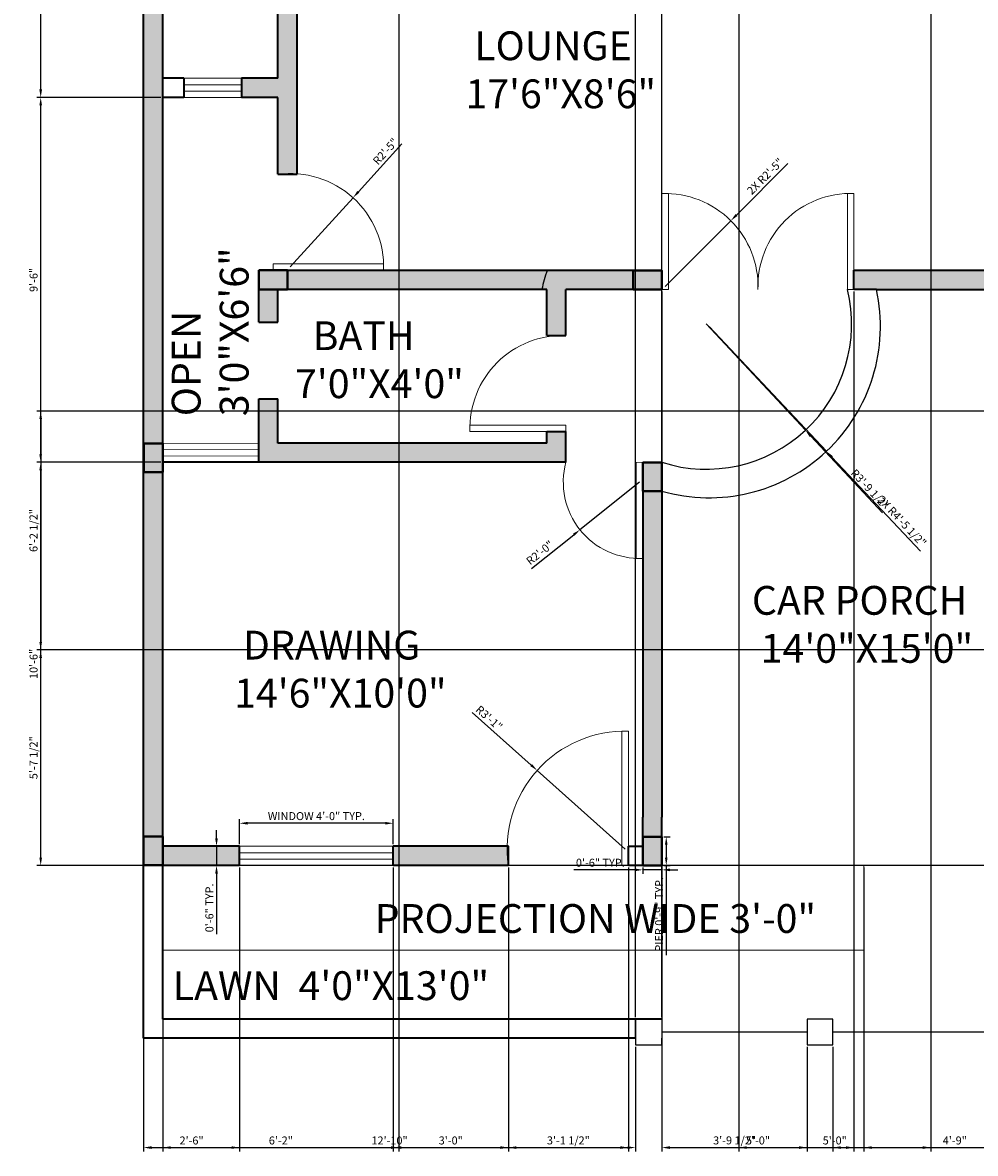
# Model space of a CAD drawing. Units: inches. Extents: x 5276 to 5736, y 3292 to 3966.
# Tile 1 of 3: x 5276 to 5574, y 3292 to 3646. Entities that reach past the tile are written whole.
import ezdxf

# ---------------------------------------------------------------- set-up
doc = ezdxf.new("R2010")
doc.units = ezdxf.units.IN
for name, color, linetype, lineweight in [('A-ANNO-DIMS', 2, 'Continuous', 18), ('A-ANNO-TEXT', 7, 'Continuous', 18), ('A-AREA-IDEN', 7, 'Continuous', 18), ('A-COLS', 7, 'Continuous', 40), ('A-DOOR', 3, 'Continuous', 18), ('A-FLOR', 7, 'Continuous', 25), ('A-GLAZ', 4, 'Continuous', 18), ('A-ROOF', 9, 'Continuous', 18), ('A-SITE-GATE', 7, 'Continuous', 25), ('A-WALL', 7, 'Continuous', 35)]:
    doc.layers.add(name, color=color, linetype=linetype, lineweight=lineweight)
doc.layers.add('A-COLS-PATT', color=244, linetype='Continuous', lineweight=13, true_color=0x991b1e)
doc.layers.add('A-WALL-PATT', color=141, linetype='Continuous', lineweight=13, true_color=0xadddf7)
doc.styles.get("Standard").update_dxf_attribs({"font": 'arial.ttf'})
doc.dimstyles.new('ISO-25', dxfattribs={"dimtxt": 2.5, "dimasz": 2.5, "dimexe": 1.25, "dimexo": 0.625, "dimtad": 1, "dimlunit": 3, "dimtxsty": 'Standard', "dimcen": 2.5, "dimadec": 0, "dimazin": 0, "dimtfac": 1, "dimtmove": 0, "dimatfit": 3, "dimfxl": 1, "dimarcsym": 0})

# ---------------------------------------------------------------- blocks, each defined once
blk = doc.blocks.new('PIER-6X9')
for p, q in [((0, 9), (6, 9)), ((0, 0), (0, 9)), ((6, 9), (6, 0)), ((6, 0), (0, 0))]:
    blk.add_line(p, q)
blk = doc.blocks.new('DOOR-SWING-30')
for p, q in [((0, 30), (-2, 30)), ((-2, 30), (-2, 0)), ((0, 0), (0, 30)), ((-2, 0), (0, 0))]:
    blk.add_line(p, q)
blk.add_arc((-1, 1), 29.02, 88.0251, 181.9749)
blk = doc.blocks.new('WINDOW-48X6')
for p, q in [((0, 6), (0, 0)), ((48, 6), (0, 6)), ((48, 4), (0, 4)), ((48, 0), (48, 6)), ((48, 2), (0, 2)), ((0, 0), (48, 0))]:
    blk.add_line(p, q)
blk = doc.blocks.new('*D22')
at = {"layer": 'A-ANNO-DIMS', "color": 0, "lineweight": -2, "transparency": 16777216}
for p, q in [((5476.74, 3391.24), (5478.72, 3391.24)), ((5477.47, 3388.74), (5477.47, 3384.74)), ((5476.74, 3382.24), (5478.72, 3382.24)), ((5477.47, 3382.24), (5477.47, 3354.25))]:
    blk.add_line(p, q, dxfattribs=at)
at = {"layer": 'A-ANNO-DIMS', "color": 0, "transparency": 16777216}
for points in [[(5477.05, 3388.74), (5477.88, 3388.74), (5477.47, 3391.24)], [(5477.05, 3384.74), (5477.88, 3384.74), (5477.47, 3382.24)]]:
    blk.add_solid(points, dxfattribs=at)
at = {"layer": 'Defpoints', "color": 0, "transparency": 16777216}
for p in [(5476.12, 3391.24), (5476.12, 3382.24), (5477.47, 3382.24)]:
    blk.add_point(p, dxfattribs=at)
at = {"layer": 'A-ANNO-DIMS', "color": 0, "transparency": 16777216, "insert": (5475.56, 3367), "char_height": 2.5, "attachment_point": 5, "rotation": 90}
blk.add_mtext('PIER 0\'-9" TYP.', dxfattribs=at)
blk = doc.blocks.new('*D23')
at = {"layer": 'A-ANNO-DIMS', "color": 0, "lineweight": -2, "transparency": 16777216}
for p, q in [((5467.62, 3380.89), (5448.63, 3380.89)), ((5470.12, 3381.61), (5470.12, 3379.64)), ((5476.12, 3380.89), (5470.12, 3380.89)), ((5476.12, 3381.61), (5476.12, 3379.64)), ((5478.62, 3380.89), (5481.12, 3380.89))]:
    blk.add_line(p, q, dxfattribs=at)
at = {"layer": 'A-ANNO-DIMS', "color": 0, "transparency": 16777216}
for points in [[(5467.62, 3381.31), (5467.62, 3380.47), (5470.12, 3380.89)], [(5478.62, 3381.31), (5478.62, 3380.47), (5476.12, 3380.89)]]:
    blk.add_solid(points, dxfattribs=at)
at = {"layer": 'Defpoints', "color": 0, "transparency": 16777216}
for p in [(5470.12, 3382.24), (5476.12, 3382.24), (5470.12, 3380.89)]:
    blk.add_point(p, dxfattribs=at)
at = {"layer": 'A-ANNO-DIMS', "color": 0, "transparency": 16777216, "insert": (5456.87, 3382.79), "char_height": 2.5, "attachment_point": 5}
blk.add_mtext('0\'-6" TYP.', dxfattribs=at)
blk = doc.blocks.new('*D28')
at = {"layer": 'A-ANNO-DIMS', "color": 0, "lineweight": -2, "transparency": 16777216}
for p, q in [((5344.13, 3388.87), (5344.13, 3396.7)), ((5392.13, 3388.87), (5392.13, 3396.7)), ((5389.63, 3395.45), (5346.63, 3395.45))]:
    blk.add_line(p, q, dxfattribs=at)
at = {"layer": 'A-ANNO-DIMS', "color": 0, "transparency": 16777216}
for points in [[(5346.63, 3395.87), (5346.63, 3395.03), (5344.13, 3395.45)], [(5389.63, 3395.87), (5389.63, 3395.03), (5392.13, 3395.45)]]:
    blk.add_solid(points, dxfattribs=at)
at = {"layer": 'Defpoints', "color": 0, "transparency": 16777216}
for p in [(5344.13, 3395.45), (5344.13, 3388.25), (5392.13, 3388.25)]:
    blk.add_point(p, dxfattribs=at)
at = {"layer": 'A-ANNO-DIMS', "color": 0, "transparency": 16777216, "insert": (5368.13, 3397.37), "char_height": 2.5, "attachment_point": 5}
blk.add_mtext('WINDOW 4\'-0" TYP.', dxfattribs=at)
blk = doc.blocks.new('*D29')
at = {"layer": 'A-ANNO-DIMS', "color": 0, "lineweight": -2, "transparency": 16777216}
for p, q in [((5336.93, 3390.75), (5336.93, 3393.25)), ((5343.5, 3388.25), (5335.68, 3388.25)), ((5336.93, 3388.25), (5336.93, 3382.25)), ((5343.5, 3382.25), (5335.68, 3382.25)), ((5336.93, 3379.75), (5336.93, 3360.76))]:
    blk.add_line(p, q, dxfattribs=at)
at = {"layer": 'A-ANNO-DIMS', "color": 0, "transparency": 16777216}
for points in [[(5336.51, 3390.75), (5337.34, 3390.75), (5336.93, 3388.25)], [(5336.51, 3379.75), (5337.34, 3379.75), (5336.93, 3382.25)]]:
    blk.add_solid(points, dxfattribs=at)
at = {"layer": 'Defpoints', "color": 0, "transparency": 16777216}
for p in [(5344.13, 3388.25), (5336.93, 3382.25), (5344.13, 3382.25)]:
    blk.add_point(p, dxfattribs=at)
at = {"layer": 'A-ANNO-DIMS', "color": 0, "transparency": 16777216, "insert": (5335.03, 3369), "char_height": 2.5, "attachment_point": 5, "rotation": 90}
blk.add_mtext('0\'-6" TYP.', dxfattribs=at)
blk = doc.blocks.new('*D30')
at = {"layer": 'A-ANNO-DIMS', "color": 0, "lineweight": -2, "transparency": 16777216}
for p, q in [((5314.13, 3327.62), (5314.13, 3292.85)), ((5467.88, 3325.62), (5467.88, 3292.85)), ((5316.63, 3294.1), (5465.38, 3294.1))]:
    blk.add_line(p, q, dxfattribs=at)
at = {"layer": 'A-ANNO-DIMS', "color": 0, "transparency": 16777216}
for points in [[(5316.63, 3294.52), (5316.63, 3293.68), (5314.13, 3294.1)], [(5465.38, 3294.52), (5465.38, 3293.68), (5467.88, 3294.1)]]:
    blk.add_solid(points, dxfattribs=at)
at = {"layer": 'Defpoints', "color": 0, "transparency": 16777216}
for p in [(5314.13, 3328.25), (5467.88, 3326.25), (5467.88, 3294.1)]:
    blk.add_point(p, dxfattribs=at)
at = {"layer": 'A-ANNO-DIMS', "color": 0, "transparency": 16777216, "insert": (5391, 3296), "char_height": 2.5, "attachment_point": 5}
blk.add_mtext('12\'-10"', dxfattribs=at)
blk = doc.blocks.new('*D31')
at = {"layer": 'A-ANNO-DIMS', "color": 0, "lineweight": -2, "transparency": 16777216}
for p, q in [((5476.13, 3325.62), (5476.13, 3292.85)), ((5521.5, 3325.62), (5521.5, 3292.85)), ((5478.63, 3294.1), (5519, 3294.1))]:
    blk.add_line(p, q, dxfattribs=at)
at = {"layer": 'A-ANNO-DIMS', "color": 0, "transparency": 16777216}
for points in [[(5478.63, 3294.52), (5478.63, 3293.68), (5476.13, 3294.1)], [(5519, 3294.52), (5519, 3293.68), (5521.5, 3294.1)]]:
    blk.add_solid(points, dxfattribs=at)
at = {"layer": 'Defpoints', "color": 0, "transparency": 16777216}
for p in [(5476.13, 3326.25), (5521.5, 3326.25), (5521.5, 3294.1)]:
    blk.add_point(p, dxfattribs=at)
at = {"layer": 'A-ANNO-DIMS', "color": 0, "transparency": 16777216, "insert": (5498.82, 3296.02), "char_height": 2.5, "attachment_point": 5}
blk.add_mtext('3\'-9 1/2"', dxfattribs=at)
blk = doc.blocks.new('*D32')
at = {"layer": 'A-ANNO-DIMS', "color": 0, "lineweight": -2, "transparency": 16777216}
for p, q in [((5529.5, 3325.62), (5529.5, 3292.85)), ((5672.13, 3325.62), (5672.13, 3292.85)), ((5532, 3294.1), (5669.63, 3294.1))]:
    blk.add_line(p, q, dxfattribs=at)
at = {"layer": 'A-ANNO-DIMS', "color": 0, "transparency": 16777216}
for points in [[(5532, 3294.52), (5532, 3293.68), (5529.5, 3294.1)], [(5669.63, 3294.52), (5669.63, 3293.68), (5672.13, 3294.1)]]:
    blk.add_solid(points, dxfattribs=at)
at = {"layer": 'Defpoints', "color": 0, "transparency": 16777216}
for p in [(5529.5, 3326.25), (5672.13, 3326.25), (5672.13, 3294.1)]:
    blk.add_point(p, dxfattribs=at)
at = {"layer": 'A-ANNO-DIMS', "color": 0, "transparency": 16777216, "insert": (5600.82, 3296.02), "char_height": 2.5, "attachment_point": 5}
blk.add_mtext('11\'-10 1/2"', dxfattribs=at)
blk = doc.blocks.new('*D33')
at = {"layer": 'A-ANNO-DIMS', "color": 0, "lineweight": -2, "transparency": 16777216}
for p, q in [((5467.88, 3334.87), (5467.88, 3961.65)), ((5476.13, 3334.87), (5476.13, 3961.65)), ((5470.38, 3960.4), (5473.63, 3960.4)), ((5476.13, 3960.4), (5492.35, 3960.4))]:
    blk.add_line(p, q, dxfattribs=at)
at = {"layer": 'A-ANNO-DIMS', "color": 0, "transparency": 16777216}
for points in [[(5470.38, 3960.82), (5470.38, 3959.98), (5467.88, 3960.4)], [(5473.63, 3960.82), (5473.63, 3959.98), (5476.13, 3960.4)]]:
    blk.add_solid(points, dxfattribs=at)
at = {"layer": 'Defpoints', "color": 0, "transparency": 16777216}
for p in [(5476.13, 3960.4), (5467.88, 3334.25), (5476.13, 3334.25)]:
    blk.add_point(p, dxfattribs=at)
at = {"layer": 'A-ANNO-DIMS', "color": 0, "transparency": 16777216, "insert": (5485.49, 3962.32), "char_height": 2.5, "attachment_point": 5}
blk.add_mtext('0\'-8 1/2"', dxfattribs=at)
blk = doc.blocks.new('*D36')
at = {"layer": 'A-ANNO-DIMS', "color": 0, "lineweight": -2, "transparency": 16777216}
for p, q in [((5319.5, 3508.25), (5280.73, 3508.25)), ((5281.98, 3384.75), (5281.98, 3505.75)), ((5319.5, 3382.25), (5280.73, 3382.25))]:
    blk.add_line(p, q, dxfattribs=at)
at = {"layer": 'A-ANNO-DIMS', "color": 0, "transparency": 16777216}
for points in [[(5281.56, 3505.75), (5282.39, 3505.75), (5281.98, 3508.25)], [(5281.56, 3384.75), (5282.39, 3384.75), (5281.98, 3382.25)]]:
    blk.add_solid(points, dxfattribs=at)
at = {"layer": 'Defpoints', "color": 0, "transparency": 16777216}
for p in [(5281.98, 3508.25), (5320.13, 3508.25), (5320.13, 3382.25)]:
    blk.add_point(p, dxfattribs=at)
at = {"layer": 'A-ANNO-DIMS', "color": 0, "transparency": 16777216, "insert": (5280.08, 3445.25), "char_height": 2.5, "attachment_point": 5, "rotation": 90}
blk.add_mtext('10\'-6"', dxfattribs=at)
blk = doc.blocks.new('*D37')
at = {"layer": 'A-ANNO-DIMS', "color": 0, "lineweight": -2, "transparency": 16777216}
for p, q in [((5319.5, 3622.25), (5280.73, 3622.25)), ((5281.98, 3510.75), (5281.98, 3619.75)), ((5319.5, 3508.25), (5280.73, 3508.25))]:
    blk.add_line(p, q, dxfattribs=at)
at = {"layer": 'A-ANNO-DIMS', "color": 0, "transparency": 16777216}
for points in [[(5281.56, 3619.75), (5282.39, 3619.75), (5281.98, 3622.25)], [(5281.56, 3510.75), (5282.39, 3510.75), (5281.98, 3508.25)]]:
    blk.add_solid(points, dxfattribs=at)
at = {"layer": 'Defpoints', "color": 0, "transparency": 16777216}
for p in [(5281.98, 3622.25), (5320.13, 3622.25), (5320.13, 3508.25)]:
    blk.add_point(p, dxfattribs=at)
at = {"layer": 'A-ANNO-DIMS', "color": 0, "transparency": 16777216, "insert": (5280.08, 3565.25), "char_height": 2.5, "attachment_point": 5, "rotation": 90}
blk.add_mtext('9\'-6"', dxfattribs=at)
blk = doc.blocks.new('*D38')
at = {"layer": 'A-ANNO-DIMS', "color": 0, "lineweight": -2, "transparency": 16777216}
for p, q in [((5319.5, 3730.25), (5280.73, 3730.25)), ((5281.98, 3624.75), (5281.98, 3727.75)), ((5319.5, 3622.25), (5280.73, 3622.25))]:
    blk.add_line(p, q, dxfattribs=at)
at = {"layer": 'A-ANNO-DIMS', "color": 0, "transparency": 16777216}
for points in [[(5281.56, 3727.75), (5282.39, 3727.75), (5281.98, 3730.25)], [(5281.56, 3624.75), (5282.39, 3624.75), (5281.98, 3622.25)]]:
    blk.add_solid(points, dxfattribs=at)
at = {"layer": 'Defpoints', "color": 0, "transparency": 16777216}
for p in [(5281.98, 3730.25), (5320.13, 3730.25), (5320.13, 3622.25)]:
    blk.add_point(p, dxfattribs=at)
at = {"layer": 'A-ANNO-DIMS', "color": 0, "transparency": 16777216, "insert": (5280.08, 3676.25), "char_height": 2.5, "attachment_point": 5, "rotation": 90}
blk.add_mtext('9\'-0"', dxfattribs=at)
blk = doc.blocks.new('*D41')
at = {"layer": 'A-ANNO-DIMS', "color": 0, "lineweight": -2, "transparency": 16777216}
for p, q in [((5476.13, 3382.87), (5476.13, 3961.65)), ((5596.12, 3382.87), (5596.12, 3961.65)), ((5478.63, 3960.4), (5593.62, 3960.4))]:
    blk.add_line(p, q, dxfattribs=at)
at = {"layer": 'A-ANNO-DIMS', "color": 0, "transparency": 16777216}
for points in [[(5478.63, 3960.82), (5478.63, 3959.98), (5476.13, 3960.4)], [(5593.62, 3960.82), (5593.62, 3959.98), (5596.12, 3960.4)]]:
    blk.add_solid(points, dxfattribs=at)
at = {"layer": 'Defpoints', "color": 0, "transparency": 16777216}
for p in [(5596.12, 3960.4), (5476.13, 3382.25), (5596.12, 3382.25)]:
    blk.add_point(p, dxfattribs=at)
at = {"layer": 'A-ANNO-DIMS', "color": 0, "transparency": 16777216, "insert": (5536.12, 3962.3), "char_height": 2.5, "attachment_point": 5}
blk.add_mtext('10\'-0"', dxfattribs=at)
blk = doc.blocks.new('*D42')
at = {"layer": 'A-ANNO-DIMS', "color": 0, "lineweight": -2, "transparency": 16777216}
for p, q in [((5539.19, 3381.62), (5539.19, 3292.85)), ((5596.12, 3381.62), (5596.12, 3292.85)), ((5541.69, 3294.1), (5593.62, 3294.1))]:
    blk.add_line(p, q, dxfattribs=at)
at = {"layer": 'A-ANNO-DIMS', "color": 0, "transparency": 16777216}
for points in [[(5541.69, 3294.52), (5541.69, 3293.68), (5539.19, 3294.1)], [(5593.62, 3294.52), (5593.62, 3293.68), (5596.12, 3294.1)]]:
    blk.add_solid(points, dxfattribs=at)
at = {"layer": 'Defpoints', "color": 0, "transparency": 16777216}
for p in [(5539.19, 3382.25), (5596.12, 3382.25), (5596.12, 3294.1)]:
    blk.add_point(p, dxfattribs=at)
at = {"layer": 'A-ANNO-DIMS', "color": 0, "transparency": 16777216, "insert": (5567.65, 3296), "char_height": 2.5, "attachment_point": 5}
blk.add_mtext('4\'-9"', dxfattribs=at)
blk = doc.blocks.new('*D45')
at = {"layer": 'A-ANNO-DIMS', "color": 0, "lineweight": -2, "transparency": 16777216}
for p, q in [((5639.55, 3524.24), (5280.73, 3524.24)), ((5281.98, 3521.74), (5281.98, 3452.12)), ((5641.55, 3449.62), (5280.73, 3449.62))]:
    blk.add_line(p, q, dxfattribs=at)
at = {"layer": 'A-ANNO-DIMS', "color": 0, "transparency": 16777216}
for points in [[(5281.56, 3521.74), (5282.39, 3521.74), (5281.98, 3524.24)], [(5281.56, 3452.12), (5282.39, 3452.12), (5281.98, 3449.62)]]:
    blk.add_solid(points, dxfattribs=at)
at = {"layer": 'Defpoints', "color": 0, "transparency": 16777216}
for p in [(5640.17, 3524.24), (5281.98, 3449.62), (5642.17, 3449.62)]:
    blk.add_point(p, dxfattribs=at)
at = {"layer": 'A-ANNO-DIMS', "color": 0, "transparency": 16777216, "insert": (5280.06, 3486.93), "char_height": 2.5, "attachment_point": 5, "rotation": 90}
blk.add_mtext('6\'-2 1/2"', dxfattribs=at)
blk = doc.blocks.new('*D46')
at = {"layer": 'A-ANNO-DIMS', "color": 0, "lineweight": -2, "transparency": 16777216}
for p, q in [((5595.49, 3449.62), (5280.73, 3449.62)), ((5281.98, 3384.75), (5281.98, 3447.12)), ((5595.49, 3382.25), (5280.73, 3382.25))]:
    blk.add_line(p, q, dxfattribs=at)
at = {"layer": 'A-ANNO-DIMS', "color": 0, "transparency": 16777216}
for points in [[(5281.56, 3447.12), (5282.39, 3447.12), (5281.98, 3449.62)], [(5281.56, 3384.75), (5282.39, 3384.75), (5281.98, 3382.25)]]:
    blk.add_solid(points, dxfattribs=at)
at = {"layer": 'Defpoints', "color": 0, "transparency": 16777216}
for p in [(5281.98, 3449.62), (5596.12, 3449.62), (5596.12, 3382.25)]:
    blk.add_point(p, dxfattribs=at)
at = {"layer": 'A-ANNO-DIMS', "color": 0, "transparency": 16777216, "insert": (5280.06, 3415.93), "char_height": 2.5, "attachment_point": 5, "rotation": 90}
blk.add_mtext('5\'-7 1/2"', dxfattribs=at)
blk = doc.blocks.new('*D48')
at = {"layer": 'A-ANNO-DIMS', "color": 0, "lineweight": -2, "transparency": 16777216}
for p, q in [((5314.14, 3381.68), (5314.14, 3292.85)), ((5344.13, 3381.62), (5344.13, 3292.85)), ((5316.64, 3294.1), (5341.63, 3294.1))]:
    blk.add_line(p, q, dxfattribs=at)
at = {"layer": 'A-ANNO-DIMS', "color": 0, "transparency": 16777216}
for points in [[(5316.64, 3294.52), (5316.64, 3293.68), (5314.14, 3294.1)], [(5341.63, 3294.52), (5341.63, 3293.68), (5344.13, 3294.1)]]:
    blk.add_solid(points, dxfattribs=at)
at = {"layer": 'Defpoints', "color": 0, "transparency": 16777216}
for p in [(5314.14, 3382.31), (5344.13, 3382.25), (5344.13, 3294.1)]:
    blk.add_point(p, dxfattribs=at)
at = {"layer": 'A-ANNO-DIMS', "color": 0, "transparency": 16777216, "insert": (5329.13, 3296), "char_height": 2.5, "attachment_point": 5}
blk.add_mtext('2\'-6"', dxfattribs=at)
blk = doc.blocks.new('*D49')
at = {"layer": 'A-ANNO-DIMS', "color": 0, "lineweight": -2, "transparency": 16777216}
for p, q in [((5392.13, 3381.62), (5392.13, 3292.85)), ((5428.13, 3381.62), (5428.13, 3292.85)), ((5394.63, 3294.1), (5425.63, 3294.1))]:
    blk.add_line(p, q, dxfattribs=at)
at = {"layer": 'A-ANNO-DIMS', "color": 0, "transparency": 16777216}
for points in [[(5394.63, 3294.52), (5394.63, 3293.68), (5392.13, 3294.1)], [(5425.63, 3294.52), (5425.63, 3293.68), (5428.13, 3294.1)]]:
    blk.add_solid(points, dxfattribs=at)
at = {"layer": 'Defpoints', "color": 0, "transparency": 16777216}
for p in [(5392.13, 3382.25), (5428.13, 3382.25), (5428.13, 3294.1)]:
    blk.add_point(p, dxfattribs=at)
at = {"layer": 'A-ANNO-DIMS', "color": 0, "transparency": 16777216, "insert": (5410.13, 3296), "char_height": 2.5, "attachment_point": 5}
blk.add_mtext('3\'-0"', dxfattribs=at)
blk = doc.blocks.new('*D50')
at = {"layer": 'A-ANNO-DIMS', "color": 0, "lineweight": -2, "transparency": 16777216}
for p, q in [((5428.13, 3381.62), (5428.13, 3292.85)), ((5465.63, 3381.62), (5465.63, 3292.85)), ((5430.63, 3294.1), (5463.13, 3294.1))]:
    blk.add_line(p, q, dxfattribs=at)
at = {"layer": 'A-ANNO-DIMS', "color": 0, "transparency": 16777216}
for points in [[(5430.63, 3294.52), (5430.63, 3293.68), (5428.13, 3294.1)], [(5463.13, 3294.52), (5463.13, 3293.68), (5465.63, 3294.1)]]:
    blk.add_solid(points, dxfattribs=at)
at = {"layer": 'Defpoints', "color": 0, "transparency": 16777216}
for p in [(5428.13, 3382.25), (5465.63, 3382.25), (5465.63, 3294.1)]:
    blk.add_point(p, dxfattribs=at)
at = {"layer": 'A-ANNO-DIMS', "color": 0, "transparency": 16777216, "insert": (5446.88, 3296.02), "char_height": 2.5, "attachment_point": 5}
blk.add_mtext('3\'-1 1/2"', dxfattribs=at)
blk = doc.blocks.new('*D51')
at = {"layer": 'A-ANNO-DIMS', "color": 0, "lineweight": -2, "transparency": 16777216}
for p, q in [((5476.13, 3561.62), (5476.13, 3292.85)), ((5536.13, 3561.62), (5536.13, 3292.85)), ((5478.63, 3294.1), (5533.63, 3294.1))]:
    blk.add_line(p, q, dxfattribs=at)
at = {"layer": 'A-ANNO-DIMS', "color": 0, "transparency": 16777216}
for points in [[(5478.63, 3294.52), (5478.63, 3293.68), (5476.13, 3294.1)], [(5533.63, 3294.52), (5533.63, 3293.68), (5536.13, 3294.1)]]:
    blk.add_solid(points, dxfattribs=at)
at = {"layer": 'Defpoints', "color": 0, "transparency": 16777216}
for p in [(5476.13, 3562.25), (5536.13, 3562.25), (5536.13, 3294.1)]:
    blk.add_point(p, dxfattribs=at)
at = {"layer": 'A-ANNO-DIMS', "color": 0, "transparency": 16777216, "insert": (5506.13, 3296), "char_height": 2.5, "attachment_point": 5}
blk.add_mtext('5\'-0"', dxfattribs=at)
blk = doc.blocks.new('*D53')
at = {"layer": 'A-ANNO-DIMS', "color": 0, "lineweight": -2, "transparency": 16777216}
for p, q in [((5320.13, 3867.62), (5320.13, 3292.85)), ((5393.93, 3867.62), (5393.93, 3292.85)), ((5322.63, 3294.1), (5391.43, 3294.1))]:
    blk.add_line(p, q, dxfattribs=at)
at = {"layer": 'A-ANNO-DIMS', "color": 0, "transparency": 16777216}
for points in [[(5322.63, 3294.52), (5322.63, 3293.68), (5320.13, 3294.1)], [(5391.43, 3294.52), (5391.43, 3293.68), (5393.93, 3294.1)]]:
    blk.add_solid(points, dxfattribs=at)
at = {"layer": 'Defpoints', "color": 0, "transparency": 16777216}
for p in [(5320.13, 3868.25), (5393.93, 3868.25), (5393.93, 3294.1)]:
    blk.add_point(p, dxfattribs=at)
at = {"layer": 'A-ANNO-DIMS', "color": 0, "transparency": 16777216, "insert": (5357.03, 3296), "char_height": 2.5, "attachment_point": 5}
blk.add_mtext('6\'-2"', dxfattribs=at)
blk = doc.blocks.new('*D54')
at = {"layer": 'A-ANNO-DIMS', "color": 0, "lineweight": -2, "transparency": 16777216}
for p, q in [((5500.14, 3867.62), (5500.14, 3292.85)), ((5560.13, 3867.62), (5560.13, 3292.85)), ((5502.64, 3294.1), (5557.63, 3294.1))]:
    blk.add_line(p, q, dxfattribs=at)
at = {"layer": 'A-ANNO-DIMS', "color": 0, "transparency": 16777216}
for points in [[(5502.64, 3294.52), (5502.64, 3293.68), (5500.14, 3294.1)], [(5557.63, 3294.52), (5557.63, 3293.68), (5560.13, 3294.1)]]:
    blk.add_solid(points, dxfattribs=at)
at = {"layer": 'Defpoints', "color": 0, "transparency": 16777216}
for p in [(5500.14, 3868.25), (5560.13, 3868.25), (5560.13, 3294.1)]:
    blk.add_point(p, dxfattribs=at)
at = {"layer": 'A-ANNO-DIMS', "color": 0, "transparency": 16777216, "insert": (5530.13, 3296), "char_height": 2.5, "attachment_point": 5}
blk.add_mtext('5\'-0"', dxfattribs=at)
blk = doc.blocks.new('*D57')
at = {"layer": 'A-ANNO-DIMS', "color": 0, "lineweight": -2, "transparency": 16777216}
for p, q in [((5490.86, 3550.71), (5527.53, 3511.69)), ((5556.9, 3480.44), (5529.24, 3509.87))]:
    blk.add_line(p, q, dxfattribs=at)
at = {"layer": 'A-ANNO-DIMS', "color": 0, "transparency": 16777216}
blk.add_solid([(5529.54, 3510.16), (5528.94, 3509.58), (5527.53, 3511.69)], dxfattribs=at)
at = {"layer": 'Defpoints', "color": 0, "transparency": 16777216}
for p in [(5490.86, 3550.71), (5527.53, 3511.69)]:
    blk.add_point(p, dxfattribs=at)
at = {"layer": 'A-ANNO-DIMS', "color": 0, "transparency": 16777216, "insert": (5550.93, 3489.6), "char_height": 2.5, "attachment_point": 5, "rotation": 313.2247}
blk.add_mtext('2X R4\'-5 1/2"', dxfattribs=at)
blk = doc.blocks.new('*D59')
at = {"layer": 'A-ANNO-DIMS', "color": 0, "lineweight": -2, "transparency": 16777216}
for p, q in [((5489.99, 3551.51), (5520.94, 3518.26)), ((5545, 3492.42), (5522.64, 3516.43))]:
    blk.add_line(p, q, dxfattribs=at)
at = {"layer": 'A-ANNO-DIMS', "color": 0, "transparency": 16777216}
blk.add_solid([(5522.95, 3516.72), (5522.34, 3516.15), (5520.94, 3518.26)], dxfattribs=at)
at = {"layer": 'Defpoints', "color": 0, "transparency": 16777216}
for p in [(5489.99, 3551.51), (5520.94, 3518.26)]:
    blk.add_point(p, dxfattribs=at)
at = {"layer": 'A-ANNO-DIMS', "color": 0, "transparency": 16777216, "insert": (5540.92, 3499.62), "char_height": 2.5, "attachment_point": 5, "rotation": 312.9546}
blk.add_mtext('R3\'-9 1/2"', dxfattribs=at)
blk = doc.blocks.new('*D61')
at = {"layer": 'A-ANNO-DIMS', "color": 0, "lineweight": -2, "transparency": 16777216}
for p, q in [((5416.79, 3430.11), (5435.26, 3413.62)), ((5464.63, 3387.4), (5437.13, 3411.95))]:
    blk.add_line(p, q, dxfattribs=at)
at = {"layer": 'A-ANNO-DIMS', "color": 0, "transparency": 16777216}
blk.add_solid([(5435.54, 3413.93), (5434.99, 3413.31), (5437.13, 3411.95)], dxfattribs=at)
at = {"layer": 'Defpoints', "color": 0, "transparency": 16777216}
for p in [(5437.13, 3411.95), (5464.63, 3387.4)]:
    blk.add_point(p, dxfattribs=at)
at = {"layer": 'A-ANNO-DIMS', "color": 0, "transparency": 16777216, "insert": (5421.9, 3428.1), "char_height": 2.5, "attachment_point": 5, "rotation": 318.2401}
blk.add_mtext('R3\'-1"', dxfattribs=at)
blk = doc.blocks.new('*D63')
at = {"layer": 'A-ANNO-DIMS', "color": 0, "lineweight": -2, "transparency": 16777216}
for p, q in [((5515.51, 3601.61), (5499.42, 3585.51)), ((5477.14, 3563.23), (5497.65, 3583.74))]:
    blk.add_line(p, q, dxfattribs=at)
at = {"layer": 'A-ANNO-DIMS', "color": 0, "transparency": 16777216}
blk.add_solid([(5499.12, 3585.81), (5499.71, 3585.22), (5497.65, 3583.74)], dxfattribs=at)
at = {"layer": 'Defpoints', "color": 0, "transparency": 16777216}
for p in [(5497.65, 3583.74), (5477.14, 3563.23)]:
    blk.add_point(p, dxfattribs=at)
at = {"layer": 'A-ANNO-DIMS', "color": 0, "transparency": 16777216, "insert": (5508.61, 3597.4), "char_height": 2.5, "attachment_point": 5, "rotation": 45.008}
blk.add_mtext('2X R2\'-5"', dxfattribs=at)
blk = doc.blocks.new('*D64')
at = {"layer": 'A-ANNO-DIMS', "color": 0, "lineweight": -2, "transparency": 16777216}
for p, q in [((5394.81, 3607.72), (5381.26, 3592.78)), ((5359.96, 3569.3), (5379.58, 3590.93))]:
    blk.add_line(p, q, dxfattribs=at)
at = {"layer": 'A-ANNO-DIMS', "color": 0, "transparency": 16777216}
blk.add_solid([(5380.95, 3593.06), (5381.57, 3592.5), (5379.58, 3590.93)], dxfattribs=at)
at = {"layer": 'Defpoints', "color": 0, "transparency": 16777216}
for p in [(5379.58, 3590.93), (5359.96, 3569.3)]:
    blk.add_point(p, dxfattribs=at)
at = {"layer": 'A-ANNO-DIMS', "color": 0, "transparency": 16777216, "insert": (5389.95, 3605.19), "char_height": 2.5, "attachment_point": 5, "rotation": 47.7914}
blk.add_mtext('R2\'-5"', dxfattribs=at)
blk = doc.blocks.new('*D65')
at = {"layer": 'A-ANNO-DIMS', "color": 0, "lineweight": -2, "transparency": 16777216}
for p, q in [((5469.1, 3502.02), (5450.5, 3487.16)), ((5435.32, 3475.04), (5448.55, 3485.6))]:
    blk.add_line(p, q, dxfattribs=at)
at = {"layer": 'A-ANNO-DIMS', "color": 0, "transparency": 16777216}
blk.add_solid([(5448.29, 3485.93), (5448.81, 3485.28), (5450.5, 3487.16)], dxfattribs=at)
at = {"layer": 'Defpoints', "color": 0, "transparency": 16777216}
for p in [(5469.1, 3502.02), (5450.5, 3487.16)]:
    blk.add_point(p, dxfattribs=at)
at = {"layer": 'A-ANNO-DIMS', "color": 0, "transparency": 16777216, "insert": (5438.16, 3479.74), "char_height": 2.5, "attachment_point": 5, "rotation": 38.6176}
blk.add_mtext('R2\'-0"', dxfattribs=at)

msp = doc.modelspace()

# ---------------------------------------------------------------- hatches: boundary and pattern name
at = {"layer": 'A-COLS-PATT'}
h = msp.add_hatch(color=256, dxfattribs=at)
h.dxf.hatch_style = 1
h.paths.add_polyline_path([(5320.127, 3874.381), (5314.129, 3874.381), (5314.129, 3865.381), (5320.127, 3865.381)])
h.paths.add_polyline_path([(5500.127, 3874.249), (5494.136, 3874.249), (5494.136, 3865.268), (5500.127, 3865.268)])
h.paths.add_polyline_path([(5500.127, 3733.242), (5494.138, 3733.242), (5494.138, 3724.249), (5500.127, 3724.249)])
h.paths.add_polyline_path([(5569.096, 3928.221), (5560.096, 3928.221), (5560.096, 3922.249), (5560.127, 3922.249), (5566.127, 3922.23), (5566.127, 3922.249), (5569.096, 3922.249)])
h.paths.add_polyline_path([(5686.127, 3747.872), (5680.127, 3747.872), (5680.127, 3731.687), (5686.127, 3731.687)])
h.paths.add_polyline_path([(5503.112, 3676.236), (5494.127, 3676.236), (5494.127, 3670.249), (5503.112, 3670.249)])
h.paths.add_polyline_path([(5320.127, 3514.161), (5314.167, 3514.161), (5314.167, 3505.161), (5320.127, 3505.161)])
h.paths.add_polyline_path([(5320.127, 3391.305), (5314.138, 3391.305), (5314.138, 3382.305), (5320.127, 3382.305)])
h.paths.add_polyline_path([(5476.116, 3391.239), (5470.127, 3391.239), (5470.127, 3382.249), (5476.116, 3382.249)])
h.paths.add_polyline_path([(5476.1, 3508.238), (5470.127, 3508.238), (5470.127, 3499.238), (5476.1, 3499.238)])
h.paths.add_polyline_path([(5359.148, 3568.249), (5350.148, 3568.249), (5350.148, 3562.297), (5359.148, 3562.297)])
h.paths.add_polyline_path([(5476.127, 3568.222), (5467.137, 3568.222), (5467.137, 3562.249), (5476.127, 3562.249)])
h.paths.add_polyline_path([(5602.119, 3571.238), (5596.127, 3571.238), (5596.127, 3562.249), (5602.119, 3562.249)])
h.paths.add_polyline_path([(5686.112, 3571.26), (5680.127, 3571.26), (5680.127, 3568.249), (5680.112, 3562.26), (5686.112, 3562.26)])
h.paths.add_polyline_path([(5686.094, 3508.787), (5680.127, 3508.787), (5680.127, 3499.787), (5686.094, 3499.787)])
at = {"layer": 'A-WALL-PATT'}
h = msp.add_hatch(color=256, dxfattribs=at)
h.dxf.hatch_style = 1
h.paths.add_polyline_path([(5560.096, 3928.249), (5314.127, 3928.249), (5314.127, 3874.381), (5320.127, 3874.381), (5320.127, 3922.249), (5560.096, 3922.249)])
h.paths.add_polyline_path([(5500.127, 3865.268), (5494.127, 3865.268), (5494.127, 3733.242), (5500.127, 3733.242)])
h.paths.add_polyline_path([(5644.696, 3874.249), (5566.127, 3874.249), (5566.127, 3891.071), (5560.127, 3891.071), (5560.127, 3868.249), (5644.696, 3868.249)])
h.paths.add_polyline_path([(5686.127, 3928.249), (5569.096, 3928.249), (5569.096, 3922.249), (5680.127, 3922.249), (5680.127, 3874.262), (5686.127, 3874.262)])
h.paths.add_polyline_path([(5686.127, 3865.262), (5680.127, 3865.262), (5680.127, 3756.872), (5686.127, 3756.872)])
h.paths.add_polyline_path([(5393.929, 3874.249), (5320.129, 3874.249), (5320.129, 3868.249), (5393.929, 3868.249)])
h.paths.add_polyline_path([(5459.929, 3874.249), (5441.929, 3874.249), (5441.929, 3868.249), (5459.929, 3868.249)])
h.paths.add_polyline_path([(5447.929, 3730.249), (5338.127, 3730.249), (5338.127, 3724.249), (5356.127, 3724.249), (5356.127, 3628.249), (5344.74, 3628.249), (5344.74, 3622.249), (5356.127, 3622.249), (5356.127, 3598.249), (5362.127, 3598.249), (5362.127, 3724.249), (5447.929, 3724.249)])
h.paths.add_polyline_path([(5320.127, 3865.381), (5314.127, 3865.381), (5314.127, 3514.249), (5320.127, 3514.249), (5320.127, 3568.249)])
h.paths.add_polyline_path([(5686.127, 3722.687), (5680.127, 3722.687), (5680.127, 3676.249), (5503.112, 3676.249), (5503.112, 3670.249), (5596.127, 3670.249), (5596.127, 3662.687), (5602.127, 3662.687), (5602.127, 3670.249), (5680.127, 3670.249), (5680.127, 3571.26), (5686.127, 3571.26)])
h.paths.add_polyline_path([(5596.119, 3568.249), (5536.127, 3568.249), (5536.127, 3562.249), (5543.142, 3562.249), (5596.119, 3562.249)])
h.paths.add_polyline_path([(5602.127, 3632.687), (5596.127, 3632.687), (5596.127, 3571.238), (5602.127, 3571.238)])
h.paths.add_polyline_path([(5631.383, 3568.249), (5602.127, 3568.249), (5602.127, 3562.249), (5631.383, 3562.249)])
h.paths.add_polyline_path([(5680.112, 3568.249), (5661.383, 3568.249), (5661.383, 3562.249), (5680.112, 3562.249)])
h.paths.add_polyline_path([(5686.127, 3562.26), (5680.127, 3562.26), (5680.127, 3508.787), (5686.127, 3508.787)])
h.paths.add_polyline_path([(5686.127, 3499.787), (5680.127, 3499.787), (5680.127, 3391.131), (5686.127, 3391.131)])
h.paths.add_polyline_path([(5686.127, 3382.131), (5680.127, 3382.131), (5680.127, 3328.249), (5686.127, 3328.249)])
h.paths.add_polyline_path([(5320.127, 3505.161), (5314.127, 3505.161), (5314.127, 3391.305), (5320.127, 3391.305)])
h.paths.add_polyline_path([(5344.127, 3388.249), (5320.138, 3388.249), (5320.138, 3382.249), (5344.127, 3382.249)])
h.paths.add_polyline_path([(5428.127, 3388.249), (5392.127, 3388.249), (5392.127, 3382.249), (5428.127, 3382.249)])
h.paths.add_polyline_path([(5476.127, 3499.238), (5470.127, 3499.238), (5470.127, 3397.332), (5470.127, 3391.239), (5476.127, 3391.239), (5476.127, 3397.332)])
h.paths.add_polyline_path([(5446.127, 3517.875), (5440.127, 3517.875), (5440.127, 3514.249), (5356.127, 3514.249), (5356.127, 3528.065), (5350.127, 3528.065), (5350.127, 3508.249), (5446.127, 3508.249)])
h.paths.add_polyline_path([(5356.127, 3562.249), (5350.127, 3562.249), (5350.127, 3552.065), (5356.127, 3552.065)])
h.paths.add_polyline_path([(5467.137, 3568.249), (5359.148, 3568.249), (5359.148, 3562.249), (5440.127, 3562.249), (5440.127, 3547.875), (5446.127, 3547.875), (5446.127, 3562.249), (5467.137, 3562.249)])

# ---------------------------------------------------------------- linework, layer by layer
at = {"layer": 'A-DOOR'}
for p, q in [((5476.137, 3562.222), (5476.137, 3592.222)), ((5476.137, 3592.222), (5478.137, 3592.222)), ((5478.137, 3592.222), (5478.137, 3562.222)), ((5536.127, 3592.249), (5534.127, 3592.249)), ((5534.127, 3592.249), (5534.127, 3562.248)), ((5536.127, 3562.249), (5536.127, 3592.249)), ((5389.148, 3570.297), (5354.648, 3570.297)), ((5354.648, 3570.297), (5354.648, 3568.297)), ((5389.148, 3568.297), (5389.148, 3570.297)), ((5359.148, 3568.297), (5389.148, 3568.297)), ((5476.137, 3562.222), (5478.137, 3562.222)), ((5536.127, 3562.249), (5534.127, 3562.248)), ((5534.127, 3562.248), (5536.127, 3562.249)), ((5534.127, 3562.248), (5536.127, 3562.249)), ((5468.1, 3508.238), (5470.127, 3508.249)), ((5468.1, 3478.238), (5468.1, 3508.238)), ((5470.1, 3508.238), (5470.1, 3478.238)), ((5470.1, 3478.238), (5468.1, 3478.238)), ((5465.627, 3424.249), (5463.627, 3424.249)), ((5463.627, 3424.249), (5463.627, 3382.249)), ((5465.627, 3382.249), (5465.627, 3424.249)), ((5463.627, 3382.249), (5465.627, 3382.249))]:
    msp.add_line(p, q, dxfattribs=at)
for centre, radius, start, end in [((5359.96, 3569.297), 29.205, 358.03776, 97.54313), ((5477.137, 3563.227), 29.012, 358.04145, 91.9753), ((5535.127, 3563.254), 29.013, 88.02477, 182.01122), ((5469.1, 3502.02), 23.803, 164.82974, 272.40777), ((5464.627, 3387.401), 36.862, 88.44547, 188.03393)]:
    msp.add_arc(centre, radius, start, end, dxfattribs=at)
at = {"layer": 'A-FLOR'}
for centre, radius, start, end in [((5490.857, 3550.708), 53.543, 160.87601, 167.55192), ((5490.857, 3550.708), 53.543, 254.00168, 12.44808), ((5489.986, 3551.511), 45.428, 252.23698, 13.67123)]:
    msp.add_arc(centre, radius, start, end, dxfattribs=at)
at = {"layer": 'A-GLAZ'}
for p, q in [((5344.74, 3628.249), (5326.74, 3628.249)), ((5326.74, 3628.249), (5326.74, 3622.249)), ((5344.74, 3626.249), (5326.74, 3626.249)), ((5344.74, 3622.249), (5344.74, 3628.249)), ((5344.74, 3624.249), (5326.74, 3624.249)), ((5326.74, 3622.249), (5344.74, 3622.249)), ((5344.74, 3622.249), (5344.74, 3622.249)), ((5320.127, 3514.161), (5350.127, 3514.249)), ((5320.127, 3514.161), (5320.167, 3508.249)), ((5320.132, 3512.161), (5320.127, 3514.161)), ((5320.167, 3514.161), (5320.167, 3514.161)), ((5320.167, 3514.161), (5320.167, 3508.249)), ((5350.127, 3508.249), (5350.127, 3514.249)), ((5350.127, 3508.249), (5350.127, 3514.249)), ((5350.132, 3512.249), (5320.132, 3512.161)), ((5350.138, 3510.249), (5320.138, 3510.161)), ((5320.127, 3508.249), (5350.127, 3508.249)), ((5320.167, 3508.249), (5350.127, 3508.249)), ((5344.127, 3388.249), (5344.127, 3382.249))]:
    msp.add_line(p, q, dxfattribs=at)
at = {"layer": 'A-ROOF'}
for p, q in [((5596.119, 3382.249), (5539.189, 3382.249)), ((5539.189, 3382.249), (5539.189, 3355.807)), ((5539.189, 3355.807), (5320.127, 3355.807))]:
    msp.add_line(p, q, dxfattribs=at)
at = {"layer": 'A-SITE-GATE'}
for p, q in [((5467.877, 3334.249), (5467.877, 3328.249)), ((5467.877, 3334.249), (5476.127, 3334.249)), ((5467.877, 3328.249), (5467.877, 3334.249)), ((5467.877, 3334.249), (5467.877, 3326.249)), ((5476.127, 3334.249), (5476.127, 3328.249)), ((5521.504, 3334.249), (5521.504, 3328.249)), ((5521.504, 3334.249), (5521.504, 3328.249)), ((5521.504, 3334.249), (5521.504, 3326.249)), ((5529.504, 3334.249), (5521.504, 3334.249)), ((5529.504, 3326.249), (5529.504, 3334.249)), ((5476.127, 3330.249), (5521.504, 3330.249)), ((5529.504, 3330.249), (5672.127, 3330.249)), ((5467.877, 3326.249), (5476.127, 3326.249)), ((5476.127, 3326.249), (5476.127, 3328.249)), ((5521.504, 3326.249), (5529.504, 3326.249))]:
    msp.add_line(p, q, dxfattribs=at)
at = {"layer": 'A-WALL'}
for p, q in [((5314.127, 3328.249), (5314.127, 3928.249)), ((5320.127, 3568.249), (5320.127, 3922.249)), ((5356.127, 3628.249), (5356.127, 3724.249)), ((5362.127, 3598.249), (5362.127, 3724.249)), ((5326.74, 3628.249), (5320.127, 3628.249)), ((5326.74, 3628.249), (5326.74, 3622.249)), ((5356.127, 3628.249), (5344.74, 3628.249)), ((5344.74, 3628.249), (5344.74, 3622.249)), ((5326.74, 3622.249), (5320.127, 3622.249)), ((5356.127, 3622.249), (5344.74, 3622.249)), ((5356.127, 3598.249), (5356.127, 3622.249)), ((5356.127, 3598.249), (5356.127, 3622.249)), ((5356.127, 3598.249), (5362.127, 3598.249)), ((5320.127, 3334.249), (5320.127, 3568.249)), ((5350.127, 3568.249), (5476.127, 3568.249)), ((5350.127, 3552.065), (5350.127, 3568.249)), ((5476.127, 3562.249), (5476.127, 3568.249)), ((5536.127, 3562.249), (5536.127, 3568.249)), ((5536.127, 3568.249), (5596.127, 3568.249)), ((5440.127, 3562.249), (5350.127, 3562.249)), ((5356.127, 3552.065), (5356.127, 3562.249)), ((5440.127, 3547.875), (5440.127, 3562.249)), ((5446.127, 3547.875), (5446.127, 3562.249)), ((5476.127, 3562.249), (5446.127, 3562.249)), ((5543.142, 3562.249), (5536.127, 3562.249)), ((5543.142, 3562.249), (5631.383, 3562.249)), ((5350.127, 3552.065), (5356.127, 3552.065)), ((5440.127, 3547.875), (5446.127, 3547.875)), ((5350.127, 3508.249), (5350.127, 3528.065)), ((5350.127, 3528.065), (5356.127, 3528.065)), ((5356.127, 3514.249), (5356.127, 3528.065)), ((5440.127, 3514.249), (5440.127, 3517.875)), ((5440.127, 3517.875), (5446.127, 3517.875)), ((5446.127, 3508.249), (5446.127, 3517.875)), ((5440.127, 3514.249), (5356.127, 3514.249)), ((5446.127, 3508.249), (5320.127, 3508.249)), ((5470.127, 3508.249), (5470.127, 3397.332)), ((5470.127, 3508.249), (5476.127, 3508.249)), ((5476.127, 3508.249), (5476.127, 3397.332)), ((5470.127, 3382.249), (5470.127, 3397.332)), ((5476.127, 3382.249), (5476.127, 3397.332)), ((5344.127, 3388.249), (5320.127, 3388.249)), ((5344.127, 3382.249), (5344.127, 3388.249)), ((5428.127, 3388.249), (5392.127, 3388.249)), ((5392.127, 3382.249), (5392.127, 3388.249)), ((5428.127, 3382.249), (5428.127, 3388.249)), ((5465.627, 3382.249), (5465.627, 3388.249)), ((5465.627, 3388.249), (5470.127, 3388.249)), ((5344.127, 3382.249), (5320.127, 3382.249)), ((5428.127, 3382.249), (5392.127, 3382.249)), ((5470.127, 3382.249), (5465.627, 3382.249)), ((5470.127, 3382.249), (5476.127, 3382.249)), ((5476.127, 3334.249), (5320.127, 3334.249)), ((5467.877, 3328.249), (5314.127, 3328.249))]:
    msp.add_line(p, q, dxfattribs=at)

# ---------------------------------------------------------------- block references
at = {"layer": 'A-COLS'}
for p, rotation in [((5350.148, 3568.297), 269.9999999999893), ((5467.137, 3568.222), 269.9999999999933), ((5320.167, 3514.161), 180), ((5476.1, 3508.238), 180), ((5320.138, 3391.305), 180), ((5476.116, 3391.239), 180)]:
    msp.add_blockref('PIER-6X9', p, dxfattribs=dict(at, rotation=rotation))
at = {"layer": 'A-DOOR', "extrusion": (0, 0, -1), "zscale": -1, "rotation": 270.0000000000019}
msp.add_blockref('DOOR-SWING-30', (-5446.127, 3517.875), dxfattribs=at)
at = {"layer": 'A-GLAZ', "rotation": 180}
msp.add_blockref('WINDOW-48X6', (5392.127, 3388.249), dxfattribs=at)

# ---------------------------------------------------------------- texts
at = {"layer": 'A-ANNO-TEXT', "insert": (5383.611, 3370.185), "char_height": 9, "attachment_point": 1}
msp.add_mtext_dynamic_manual_height_columns(' PROJECTION WIDE 3\'-0"', width=150.09298, gutter_width=12.5, heights=[26.386], dxfattribs=at)
at = {"layer": 'A-AREA-IDEN', "char_height": 9, "attachment_point": 1}
for s, insert in [(' LOUNGE\\P17\'6"X8\'6"', (5414.722, 3642.909)), ('  BATH \\P7\'0"X4\'0"', (5361.463, 3552.307)), (' CAR PORCH\\P  14\'0"X15\'0"', (5501.486, 3469.605)), (' DRAWING\\P14\'6"X10\'0"', (5342.427, 3455.623)), (' LAWN  4\'0"X13\'0"', (5320.505, 3349.195))]:
    msp.add_mtext_dynamic_manual_height_columns(s, width=110.27411, gutter_width=12.5, heights=[0], dxfattribs=dict(at, insert=insert))
at = {"layer": 'A-AREA-IDEN', "insert": (5322.942, 3519.907), "char_height": 9, "attachment_point": 1, "rotation": 90}
msp.add_mtext_dynamic_manual_height_columns(' OPEN\\P 3\'0"X6\'6"', width=110.27411, gutter_width=12.5, heights=[0], dxfattribs=at)

# ---------------------------------------------------------------- dimensions: what is measured, and where the dimension line sits
at = {"layer": 'A-ANNO-DIMS'}
for base, p1, p2, picture, middle in [((5476.126509, 3960.399113), (5467.876509, 3334.249113), (5476.126509, 3334.249113), '*D33', (5485.487013775, 3962.316746015)), ((5596.119, 3960.399), (5476.127, 3382.249), (5596.119, 3382.249), '*D41', (5536.123, 3962.301)), ((5393.929, 3294.099), (5320.127, 3868.249), (5393.929, 3868.249), '*D53', (5357.028, 3296.001)), ((5560.127, 3294.099), (5500.136, 3868.249), (5560.127, 3868.249), '*D54', (5530.131, 3296.001)), ((5536.127, 3294.099), (5476.127, 3562.249), (5536.127, 3562.249), '*D51', (5506.127, 3296.001)), ((5344.127, 3294.099), (5314.138, 3382.305), (5344.127, 3382.249), '*D48', (5329.132, 3296.001)), ((5428.127, 3294.099), (5392.127, 3382.249), (5428.127, 3382.249), '*D49', (5410.127, 3296.001)), ((5465.627, 3294.099), (5428.127, 3382.249), (5465.627, 3382.249), '*D50', (5446.877, 3296.018)), ((5596.119, 3294.099), (5539.189, 3382.249), (5596.119, 3382.249), '*D42', (5567.654, 3296.001)), ((5467.876509, 3294.099113), (5314.126509, 3328.249113), (5467.876509, 3326.249113), '*D30', (5391.001509, 3296.000545469)), ((5521.504, 3294.099), (5476.127, 3326.249), (5521.504, 3326.249), '*D31', (5498.816, 3296.018)), ((5672.127, 3294.099), (5529.504, 3326.249), (5672.127, 3326.249), '*D32', (5600.816, 3296.017))]:
    dim = msp.add_linear_dim(base=base, p1=p1, p2=p2, dimstyle='ISO-25', override={"dimdec": 1, "dimlfac": 1, "dimrnd": 0, "dimzin": 1, "dimdsep": 46, "dimlunit": 4, "dimfrac": 2}, dxfattribs=at)
    dim.commit()
    dim.dimension.update_dxf_attribs({"geometry": picture, "text_midpoint": middle})
for base, p1, p2, picture, middle in [((5281.977, 3730.249), (5320.127, 3622.249), (5320.127, 3730.249), '*D38', (5280.075, 3676.249)), ((5281.977, 3622.249), (5320.127, 3508.249), (5320.127, 3622.249), '*D37', (5280.075, 3565.249)), ((5281.977, 3449.615), (5640.172, 3524.238), (5642.172, 3449.615), '*D45', (5280.059, 3486.927)), ((5281.977, 3508.249), (5320.127, 3382.249), (5320.127, 3508.249), '*D36', (5280.075, 3445.249)), ((5281.977, 3449.615), (5596.119, 3382.249), (5596.119, 3449.615), '*D46', (5280.059, 3415.932))]:
    dim = msp.add_linear_dim(base=base, p1=p1, p2=p2, angle=90, dimstyle='ISO-25', override={"dimdec": 1, "dimlfac": 1, "dimrnd": 0, "dimzin": 1, "dimdsep": 46, "dimlunit": 4, "dimfrac": 2}, dxfattribs=at)
    dim.commit()
    dim.dimension.update_dxf_attribs({"geometry": picture, "text_midpoint": middle})
for center, mpoint, picture, middle in [((5359.96, 3569.297), (5379.581, 3590.929), '*D64', (5391.354, 3603.908)), ((5489.986, 3551.511), (5520.941, 3518.263), '*D59', (5539.514, 3498.314)), ((5469.1, 3502.02), (5450.502, 3487.164), '*D65', (5439.343, 3478.25)), ((5464.627, 3387.401), (5437.13, 3411.951), '*D61', (5420.632, 3426.681))]:
    dim = msp.add_radius_dim(center=center, mpoint=mpoint, dimstyle='ISO-25', override={"dimdec": 1, "dimlfac": 1, "dimrnd": 0, "dimzin": 1, "dimdsep": 46, "dimlunit": 4, "dimfrac": 2}, dxfattribs=at)
    dim.commit()
    dim.dimension.update_dxf_attribs({"geometry": picture, "text_midpoint": middle, "dimtype": 164})
for center, mpoint, picture, middle in [((5477.137, 3563.227), (5497.648, 3583.744), '*D63', (5509.955, 3596.055)), ((5490.857, 3550.708), (5527.527, 3511.692), '*D57', (5549.529, 3488.283))]:
    dim = msp.add_radius_dim(center=center, mpoint=mpoint, text='2X <>', dimstyle='ISO-25', override={"dimdec": 1, "dimlfac": 1, "dimrnd": 0, "dimzin": 1, "dimdsep": 46, "dimlunit": 4, "dimfrac": 2}, dxfattribs=at)
    dim.commit()
    dim.dimension.update_dxf_attribs({"geometry": picture, "text_midpoint": middle, "dimtype": 164})
for base, p1, p2, angle, text, picture, middle in [((5344.127, 3395.449), (5392.127, 3388.249), (5344.127, 3388.249), 180, 'WINDOW <> TYP.', '*D28', (5368.127, 3397.368)), ((5336.927, 3382.249), (5344.127, 3388.249), (5344.127, 3382.249), 270, '<> TYP.', '*D29', (5335.025, 3369.005)), ((5477.466, 3382.239), (5476.116, 3391.239), (5476.116, 3382.239), 270, 'PIER <> TYP.', '*D22', (5475.564, 3366.996)), ((5470.116, 3380.889), (5476.116, 3382.239), (5470.116, 3382.239), 180, '<> TYP.', '*D23', (5456.871, 3382.79))]:
    dim = msp.add_linear_dim(base=base, p1=p1, p2=p2, angle=angle, text=text, dimstyle='ISO-25', override={"dimdec": 1, "dimlfac": 1, "dimrnd": 0, "dimzin": 1, "dimdsep": 46, "dimlunit": 4, "dimfrac": 2}, dxfattribs=at)
    dim.commit()
    dim.dimension.update_dxf_attribs({"geometry": picture, "text_midpoint": middle})

doc.saveas('drawing.dxf')
